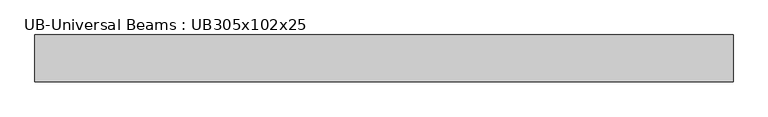
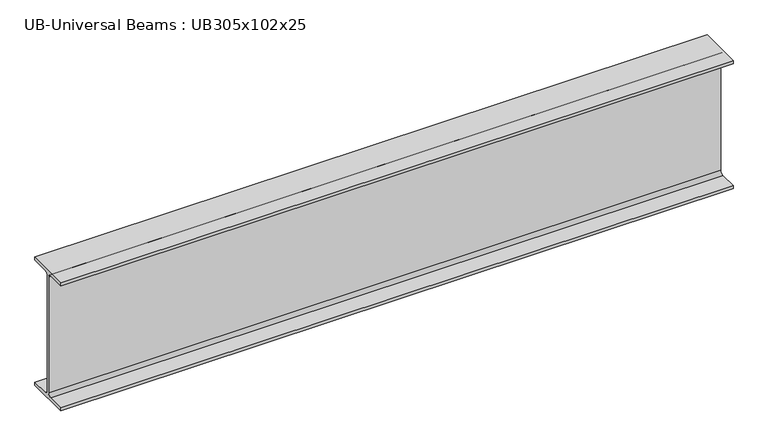
"""IFC4 building model written with IfcOpenShell, lengths in millimetres: beam geometry, UB-Universal Beams : UB305x102x25."""

from ifc_helpers import new_model, si_unit, point, frame, frame_2d, origin, place, context, project, spatial, polyline, circle_curve, trimmed, segment, composite_curve, outline, extrude, source, transform, mapped, element, save


def ub_universal_beams_ub305x102x25_8854acc3(model_context):
    return source(origin(), model_context, "Body", "SweptSolid", [
        extrude(outline(composite_curve([segment(polyline([(50.8, -145.55), (50.8, -152.55), (-50.8, -152.55), (-50.8, -145.55), (-10.5, -145.55)]), True, "CONTINUOUS"), segment(trimmed(circle_curve(frame_2d((-10.5, -137.95)), 7.6), [point((-10.5, -145.55))], [point((-2.9, -137.95))], True, "CARTESIAN"), True, "CONTINUOUS"), segment(polyline([(-2.9, -137.95), (-2.9, 137.95)]), True, "CONTINUOUS"), segment(trimmed(circle_curve(frame_2d((-10.5, 137.95)), 7.6), [point((-2.9, 137.95))], [point((-10.5, 145.55))], True, "CARTESIAN"), True, "CONTINUOUS"), segment(polyline([(-10.5, 145.55), (-50.8, 145.55), (-50.8, 152.55), (50.8, 152.55), (50.8, 145.55), (10.5, 145.55)]), True, "CONTINUOUS"), segment(trimmed(circle_curve(frame_2d((10.5, 137.95)), 7.6), [point((10.5, 145.55))], [point((2.9, 137.95))], True, "CARTESIAN"), True, "CONTINUOUS"), segment(polyline([(2.9, 137.95), (2.9, -137.95)]), True, "CONTINUOUS"), segment(trimmed(circle_curve(frame_2d((10.5, -137.95)), 7.6), [point((2.9, -137.95))], [point((10.5, -145.55))], True, "CARTESIAN"), True, "CONTINUOUS"), segment(polyline([(10.5, -145.55), (50.8, -145.55)]), True, "CONTINUOUS")], self_intersect=False)), frame((-757.6, 0.0, 0.0), z_axis=(1.0, 0.0, 0.0), x_axis=(0.0, 1.0, 0.0)), (0.0, 0.0, 1.0), 1515.2),
    ])


if __name__ == "__main__":
    model = new_model("IFC4")
    model_context = context("Model", 3, world=origin())
    ifc_project = project(units=[si_unit("LENGTHUNIT", "METRE", prefix="MILLI")], contexts=[model_context])
    site = spatial("IfcSite", under=ifc_project)
    building = spatial("IfcBuilding", under=site)
    placement = place(None, origin())
    ub_universal_beams_ub305x102x25_shape = ub_universal_beams_ub305x102x25_8854acc3(model_context)
    element("IfcBeam", 1, ObjectType="UB-Universal Beams : UB305x102x25", at=placement, inside=building, context=model_context, shape_type="MappedRepresentation", body=[
        mapped(ub_universal_beams_ub305x102x25_shape, transform((0.0, 0.0, 0.0), x_axis=(1.0, 0.0, 0.0), y_axis=(0.0, 1.0, 0.0), z_axis=(0.0, 0.0, 1.0))),
    ])
    save(model, "model.ifc")

# Revit data of these elements
# Type "UB-Universal Beams : UB305x102x25"
#   Section Name Key = "UB305X102X25"
#   Width = 10.16 cm
#   Web Thickness = 0.58 cm
#   Web Fillet = 0.76 cm
#   Warping Constant = 27300.0 cm⁶
#   Torsional Moment of Inertia = 4.77 cm⁴
#   Section Area = 31.6 cm²
#   Plastic Modulus weak axis = 39.0 cm³
#   Plastic Modulus strong axis = 342.0 cm³
#   Nominal Weight = 24.7999 kgf/m
#   Moment of Inertia weak axis = 123.00 cm⁴
#   Moment of Inertia strong axis = 4455.00 cm⁴
#   Height = 30.51 cm
#   Flange Thickness = 0.7 cm
#   Elastic Modulus weak axis = 24.2 cm³
#   Elastic Modulus strong axis = 292.0 cm³
#   Centroid Vertical = 15.255 cm
#   Centroid Horizontal = 5.08 cm
#   Bolt Spacing = 5.4 cm
#   Length [instance default] = 1.5 m
#   Structural Material [instance default] = Metal - Steel 43-275
#   Type Comments = ""
#   Assembly Code = ""
# Element 1 (IfcBeam, "UB-Universal Beams : UB305x102x25")
#   Materials on its faces: "Metal - Steel 43-275"
# Materials
#   "Metal - Steel 43-275": class "Metal", colour RGB 247 247 247, transparency 0, Cost = 0
